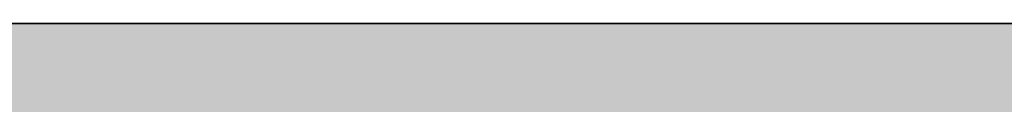
# Model space of a CAD drawing. Units: inches. Extents: x 2091 to 2899, y 967 to 2217.
# Tile 50 of 256: x 2212.145669 to 2212.151167, y 1099.918608 to 1099.919059. Entities that reach past the tile are written whole.
import ezdxf

# ---------------------------------------------------------------- set-up
doc = ezdxf.new("R2010")
doc.units = ezdxf.units.IN
doc.layers.add('A-WALL-PATT', color=141, linetype='Continuous', lineweight=13, true_color=0xadddf7)
doc.layers.add('L-SITE-WALL', color=7, linetype='Continuous', lineweight=35)

msp = doc.modelspace()

# ---------------------------------------------------------------- hatches: boundary and pattern name
at = {"layer": 'A-WALL-PATT'}
h = msp.add_hatch(color=256, dxfattribs=at)
h.dxf.hatch_style = 1
h.paths.add_polyline_path([(2212.1436027, 1941.4190588), (2387.6436027, 1941.4190588), (2387.6436027, 1824.4190588), (2392.1436027, 1824.4190588), (2392.1436027, 1941.4190588), (2609.6436027, 1941.4190588), (2609.6436027, 1825.9190588), (2614.1436027, 1825.9190588), (2614.1436027, 1941.4190588), (2794.1436027, 1941.4190588), (2794.1436027, 1928.7621663), (2803.1436027, 1928.7621663), (2803.1436027, 2050.9190588), (2203.1436027, 2050.9190588), (2203.1436027, 1900.7578592), (2212.1436027, 1900.7578592)])
h.paths.add_polyline_path([(2212.1436027, 1945.9190588), (2212.1436027, 2041.9190588), (2794.1436027, 2041.9190588), (2794.1436027, 1945.9190588), (2402.2482445, 1945.9190588), (2401.1024337, 1945.7758325), (2398.7024337, 1945.7758325)], flags=16)
h.paths.add_polyline_path([(2230.2298609, 1948.0627926), (2227.3498609, 1949.5027926), (2225.9098609, 1951.9027926), (2223.9898609, 1952.8627926), (2223.0298609, 1955.2627926), (2222.0698609, 1959.5827926), (2222.0698609, 1963.4227926), (2223.0298609, 1965.6627926), (2223.9898609, 1965.3427926), (2225.58591, 1963.860747), (2226.9115333, 1964.9572589), (2226.9488609, 1965.9387926), (2227.7783187, 1966.9521426), (2228.1999161, 1968.8787044), (2230.7098609, 1964.8627926), (2233.5898609, 1966.3027926), (2233.607309, 1966.3318728), (2233.7726595, 1964.9382048), (2234.6338015, 1963.6764729), (2235.0298609, 1963.9027926), (2236.2820348, 1965.5723578), (2235.9898609, 1962.9427926), (2237.9545121, 1957.5400019), (2238.3898609, 1957.9027926), (2239.2158609, 1960.3057926), (2238.6545655, 1966.3849599), (2238.6927918, 1966.4380694), (2238.8405779, 1967.4997069), (2238.7802908, 1967.6874864), (2238.8805378, 1967.7867629), (2238.6668609, 1966.2517926), (2239.2158609, 1960.3057926), (2238.3898609, 1957.9027926), (2236.9498609, 1956.7027926), (2234.5498609, 1949.9827926)], flags=0)
h.paths.add_polyline_path([(2278.0119735, 1948.0627926), (2276.4964266, 1947.8733492), (2275.8498328, 1947.6886081), (2274.6519735, 1947.1027926)], flags=0)
h.paths.add_polyline_path([(2269.8519735, 1955.7427926), (2268.2761762, 1956.6293287), (2270.8673022, 1956.3483982), (2269.3719735, 1958.1427926), (2268.7149641, 1959.1923253), (2270.5698328, 1958.7286081), (2268.5807252, 1961.9060872), (2270.8119735, 1960.8918835), (2270.8119735, 1963.4227926), (2271.3933148, 1964.7792556), (2270.2917623, 1966.1561963), (2271.7719735, 1965.6627926), (2272.1413868, 1966.5247568), (2273.9298328, 1965.9286081), (2275.6303855, 1968.054299), (2276.331938, 1966.72186), (2276.5204313, 1966.9521426), (2276.9420286, 1968.8787044), (2277.7342926, 1967.6110821), (2278.1398879, 1969.4645199), (2279.6591239, 1967.0337425), (2280.4119735, 1966.7827926), (2280.9493019, 1967.5887851), (2281.6098328, 1967.3686081), (2282.1332658, 1968.1537576), (2282.3492351, 1966.3334449), (2282.3498491, 1966.3325853), (2283.40755, 1968.0954201), (2283.7126314, 1965.5240203), (2284.3202211, 1964.6337894), (2284.5118085, 1964.8892393), (2284.2349735, 1965.7047926), (2284.500472, 1967.3189584), (2284.9079444, 1965.4174205), (2285.3963134, 1966.0685791), (2285.4328328, 1966.2906081), (2285.4733384, 1966.1712791), (2286.3539194, 1967.345387), (2286.2220067, 1966.1581734), (2287.6634921, 1968.0801538), (2287.7139735, 1968.4427926), (2288.4815994, 1969.0166793), (2288.5739928, 1968.7288966), (2288.9174612, 1969.0690403), (2288.6068328, 1966.8376081), (2288.9287261, 1963.3513103), (2288.9349735, 1963.3567926), (2288.9297314, 1963.3404224), (2289.015281, 1962.4138692), (2290.1112234, 1963.8751258), (2290.1328328, 1963.9426081), (2290.2176723, 1964.0170576), (2290.1112234, 1963.8751258), (2289.1558328, 1960.8916081), (2288.5940356, 1959.2572271), (2288.5719735, 1959.1027926), (2289.5319735, 1960.5427926), (2290.0119735, 1962.4627926), (2290.1918401, 1962.6426592), (2289.7698328, 1959.6886081), (2286.8898328, 1957.2886081), (2284.4898328, 1950.5686081), (2283.3146576, 1950.046308), (2283.2919735, 1949.9827926), (2280.2900585, 1948.6486081), (2281.1298328, 1948.6486081), (2282.5698328, 1948.1686081), (2283.2047262, 1948.0627926), (2278.9719735, 1948.0627926), (2276.0919735, 1949.5027926), (2274.6519735, 1951.9027926), (2272.7319735, 1952.8627926)], flags=0)
h.paths.add_polyline_path([(2271.1588684, 1958.0217654), (2272.9698328, 1955.8486081), (2272.0098328, 1960.1686081), (2272.0098328, 1964.0086081), (2272.6244258, 1965.4426583), (2274.3280226, 1963.860747), (2275.6536458, 1964.9572589), (2275.6377429, 1964.5390903), (2277.4122311, 1966.0068885), (2277.0329735, 1965.1567926), (2276.829924, 1964.9755966), (2276.7660116, 1963.2950136), (2277.4496351, 1962.6602203), (2279.4519735, 1964.8627926), (2282.3319735, 1966.3027926), (2283.5298328, 1966.8886081), (2283.2945117, 1966.7709476), (2283.9129934, 1963.8846999), (2284.8992493, 1964.4482747), (2284.7319735, 1962.9427926), (2286.6966247, 1957.5400019), (2287.1319735, 1957.9027926), (2287.5419128, 1959.0953883), (2287.7793955, 1958.4423109), (2285.6827383, 1956.6950966), (2285.8765033, 1959.7953357), (2284.7319735, 1962.9427926), (2284.8992493, 1964.4482747), (2283.9129934, 1963.8846999), (2284.2238328, 1962.4341157), (2283.4243649, 1963.6054836), (2281.6098328, 1962.5686081), (2281.1298328, 1960.1686081), (2282.0898328, 1956.3286081), (2283.0498328, 1952.9686081), (2282.5698328, 1950.5686081), (2280.1698328, 1948.6486081), (2279.883316, 1948.7918666), (2278.9719735, 1948.0627926), (2278.9719735, 1949.0227926), (2278.6723132, 1949.3973679), (2277.2898328, 1950.0886081), (2275.8498328, 1952.4886081), (2273.9298328, 1953.4486081), (2272.4898328, 1954.8886081), (2271.9216473, 1954.8886081), (2271.7719735, 1955.2627926)], flags=0)
h.paths.add_polyline_path([(2311.994146, 1955.7427926), (2312.0627174, 1955.6742211), (2312.0550999, 1955.7085002)], flags=0)
h.paths.add_polyline_path([(2331.956146, 1963.9517926), (2333.396146, 1965.3917926), (2331.077146, 1963.3567926), (2330.998603, 1963.1115166)], flags=0)
h.paths.add_polyline_path([(2310.554146, 1954.3027926), (2307.0398066, 1956.2799434), (2310.7629029, 1955.8762843), (2312.474146, 1953.8227926), (2313.434146, 1951.4227926), (2315.354146, 1950.4627926), (2316.794146, 1948.0627926), (2317.466146, 1947.7267926), (2319.3686915, 1947.9646108), (2317.754146, 1949.9827926), (2317.5695306, 1950.6104849), (2316.794146, 1951.9027926), (2314.874146, 1952.8627926), (2313.914146, 1955.2627926), (2311.514146, 1958.1427926), (2309.3754889, 1961.5591681), (2311.514146, 1960.3370783), (2311.514146, 1961.9827926), (2310.6046723, 1963.1196347), (2311.726605, 1962.4785303), (2312.4183321, 1964.09256), (2312.2559642, 1964.2955198), (2313.194146, 1963.9827926), (2313.914146, 1965.6627926), (2314.6467776, 1965.418582), (2315.354146, 1966.3027926), (2316.794146, 1967.7427926), (2316.1574354, 1966.9469043), (2317.0341105, 1965.28186), (2317.2226038, 1965.5121426), (2317.7770481, 1968.0457711), (2318.4741105, 1966.72186), (2318.6626038, 1966.9521426), (2319.0842012, 1968.8787044), (2321.2070492, 1965.4821474), (2322.1614187, 1966.9137017), (2322.554146, 1966.7827926), (2322.7859877, 1967.1305552), (2322.881646, 1966.3242926), (2323.3120408, 1965.7217399), (2323.6512889, 1965.891364), (2324.3964998, 1967.1333822), (2324.6569446, 1964.9382048), (2324.971986, 1964.476611), (2325.3872804, 1967.001499), (2325.9408127, 1964.4183481), (2327.2289286, 1966.1358361), (2327.1663199, 1965.5723578), (2328.0591386, 1966.7627827), (2328.2245759, 1966.2474864), (2329.6679714, 1967.6769101), (2329.6645759, 1967.6874864), (2329.7648229, 1967.7867629), (2329.551146, 1966.2517926), (2330.100146, 1960.3057926), (2329.3328143, 1958.0734703), (2329.3130649, 1957.935225), (2329.634146, 1958.2027926), (2330.234146, 1959.1027926), (2330.714146, 1961.0227926), (2331.034146, 1961.3427926), (2330.714146, 1959.1027926), (2329.634146, 1958.2027926), (2329.274146, 1957.6627926), (2327.7121121, 1956.3610977), (2325.434146, 1949.9827926), (2324.3337687, 1949.493736), (2323.994146, 1948.5427926), (2319.674146, 1946.6227926), (2316.794146, 1948.0627926), (2315.354146, 1950.4627926), (2313.434146, 1951.4227926)], flags=0)
h.paths.add_polyline_path([(2321.3356845, 1947.9520233), (2321.114146, 1948.0627926), (2321.114146, 1949.0227926), (2319.194146, 1951.4227926), (2316.794146, 1959.5827926), (2316.6632369, 1959.5827926), (2315.354146, 1958.1427926), (2314.394146, 1958.1427926), (2313.1483033, 1958.7090847), (2312.954146, 1959.5827926), (2312.954146, 1960.8918835), (2315.834146, 1959.5827926), (2316.6632369, 1959.5827926), (2317.3147094, 1960.2994123), (2315.0301951, 1962.420747), (2316.3558184, 1963.5172589), (2316.3723369, 1963.9516153), (2316.4701951, 1963.860747), (2317.7958184, 1964.9572589), (2317.7552187, 1963.8896871), (2319.175146, 1965.1567926), (2319.4984065, 1965.8813724), (2321.114146, 1965.3427926), (2323.2358851, 1962.3723578), (2325.6863494, 1963.7726231), (2325.5427886, 1962.4805756), (2325.1987827, 1963.4940135), (2324.4785097, 1963.0824289), (2324.9260053, 1960.9941157), (2324.0780866, 1962.2364729), (2322.4147912, 1961.2860184), (2322.074146, 1959.5827926), (2323.034146, 1955.7427926), (2323.994146, 1952.3827926), (2323.514146, 1949.9827926), (2322.1427174, 1948.8856497), (2322.074146, 1948.5427926)], flags=0)
h.paths.add_polyline_path([(2320.2074794, 1963.3374592), (2320.154146, 1963.4227926), (2320.394146, 1963.5427926)], flags=0)
h.paths.add_polyline_path([(2353.8505274, 1965.8105004), (2354.0305274, 1965.7505004), (2354.3305274, 1966.4505004), (2354.3305274, 1966.9305004)], flags=0)
h.paths.add_polyline_path([(2359.0205825, 1969.0264122), (2359.0983824, 1968.9019323), (2359.2335274, 1969.5195004), (2359.2335274, 1969.9995004)], flags=0)
h.paths.add_polyline_path([(2358.2566937, 1966.6816724), (2357.983601, 1966.3480346), (2358.211267, 1966.1461745), (2358.4104918, 1966.3895678)], flags=0)
h.paths.add_polyline_path([(2357.7684731, 1966.0587777), (2357.7321997, 1965.1049667), (2357.751047, 1965.1205565), (2357.7695274, 1965.6065004), (2357.7695274, 1966.057843)], flags=0)
h.paths.add_polyline_path([(2359.1115274, 1965.3045004), (2359.1115274, 1964.8245004), (2359.8445274, 1966.4675004), (2359.8445274, 1966.9475004)], flags=0)
h.paths.add_polyline_path([(2360.2236843, 1966.6214493), (2360.6985274, 1969.3625004), (2360.6985274, 1969.8425004), (2360.2105274, 1967.0255004), (2360.2105274, 1966.6425004)], flags=0)
h.paths.add_polyline_path([(2363.4505274, 1967.8905004), (2363.4505274, 1968.3705004), (2362.4905274, 1966.9305004), (2362.6560446, 1966.6987763)], flags=0)
h.paths.add_polyline_path([(2364.4755226, 1966.0788259), (2365.8505274, 1968.3705004), (2365.8505274, 1968.8505004), (2364.4279755, 1966.4795806)], flags=0)
h.paths.add_polyline_path([(2366.3135274, 1965.8525004), (2366.3667086, 1965.6958291), (2366.8025274, 1968.3455004), (2366.8025274, 1968.8255004)], flags=0)
h.paths.add_polyline_path([(2367.16531, 1965.8035439), (2367.2905274, 1966.9305004), (2367.2905274, 1967.4105004), (2367.1027013, 1965.7200656)], flags=0)
h.paths.add_polyline_path([(2370.0365274, 1959.9735004), (2371.0135274, 1963.0245004), (2371.0135274, 1963.5045004), (2370.0365274, 1960.4535004)], flags=0)
h.paths.add_polyline_path([(2371.6105274, 1960.2105004), (2372.5705274, 1961.6505004), (2372.5705274, 1962.1305004), (2371.8025274, 1960.9785004)], flags=0)
h.paths.add_polyline_path([(2350.8736661, 1956.0050856), (2351.9305274, 1955.8905004), (2354.4905274, 1953.3305004), (2353.8505274, 1954.9305004), (2351.4505274, 1957.8105004), (2347.9355274, 1963.4255004), (2347.9355274, 1963.9055004), (2351.4505274, 1958.2905004), (2353.7050728, 1955.5850458), (2352.8905274, 1959.2505004), (2352.8905274, 1959.7305004), (2352.8905274, 1961.9247861), (2356.7305274, 1959.7305004), (2358.454471, 1961.6268384), (2354.8105274, 1965.0105004), (2355.0308552, 1965.2859102), (2358.6910907, 1961.8871201), (2361.5305274, 1965.0105004), (2364.3764954, 1966.4334844), (2364.5243939, 1965.1869106), (2365.454468, 1963.8241807), (2365.8810728, 1964.0679549), (2365.3705274, 1966.4505004), (2365.3705274, 1966.9305004), (2366.8105274, 1960.2105004), (2366.8105274, 1959.7305004), (2366.3887092, 1952.9814095), (2367.7705274, 1956.8505004), (2368.641225, 1957.5760818), (2366.8105274, 1962.6105004), (2366.8105274, 1963.0905004), (2368.7751785, 1957.6877097), (2369.2105274, 1958.0505004), (2370.0015924, 1960.3518674), (2369.4752319, 1966.0526677), (2369.5134582, 1966.1057772), (2369.514173, 1966.1109121), (2369.4752319, 1966.5326677), (2369.5134582, 1966.5857772), (2369.614635, 1967.3125914), (2369.1825274, 1968.6585004), (2369.1825274, 1969.1385004), (2369.6009573, 1967.8351942), (2369.7012042, 1967.9344708), (2369.7179468, 1968.054743), (2370.1451758, 1968.3741448), (2369.7787075, 1968.0112238), (2369.7012042, 1967.4544708), (2370.4681613, 1968.2140038), (2369.674936, 1967.2657706), (2369.514173, 1966.1109121), (2370.0365274, 1960.4535004), (2370.0365274, 1959.9735004), (2369.441756, 1958.2431909), (2370.6505274, 1959.2505004), (2371.0458215, 1962.0175592), (2371.1305274, 1962.1305004), (2370.6505274, 1958.7705004), (2367.7705274, 1956.3705004), (2365.3705274, 1949.6505004), (2362.0790988, 1948.1876432), (2363.4505274, 1947.7305004), (2361.0505274, 1947.7305004), (2360.0905274, 1947.7305004), (2357.1038607, 1947.3571671), (2360.0905274, 1948.2105004), (2358.1705274, 1949.1705004), (2356.7305274, 1951.5705004), (2354.8105274, 1952.5305004), (2351.9305274, 1955.4105004)], flags=0)
h.paths.add_polyline_path([(2361.0505274, 1948.6905004), (2359.1305274, 1951.0905004), (2356.7305274, 1959.2505004), (2355.7705274, 1959.2505004), (2352.8905274, 1960.5595913), (2352.8905274, 1961.4447861), (2355.8905274, 1959.7305004), (2356.7305274, 1959.7305004), (2356.837194, 1959.3678337), (2361.5305274, 1964.5305004), (2363.2484221, 1965.3894478), (2364.92531, 1963.0418047), (2362.4905274, 1961.6505004), (2362.0638607, 1959.5171671), (2362.9705274, 1955.8905004), (2363.9305274, 1952.5305004), (2363.9305274, 1952.0505004), (2363.4505274, 1949.6505004), (2361.0505274, 1947.7305004)], flags=0)
h.paths.add_polyline_path([(2359.1305274, 1951.5705004), (2359.2905274, 1951.3705004), (2361.0505274, 1954.4505004), (2361.0505274, 1954.9305004)], flags=0)
h.paths.add_polyline_path([(2357.2195274, 1966.5455004), (2356.7925274, 1968.8145004), (2356.7925274, 1969.2945004), (2357.2195274, 1967.0255004)], flags=0)
h.paths.add_polyline_path([(2361.0505274, 1954.4505004), (2361.5305274, 1958.7705004), (2361.5305274, 1959.2505004), (2361.0505274, 1954.9305004)], flags=0)
h.paths.add_polyline_path([(2402.5482874, 1948.4860764), (2402.3024337, 1948.4158325), (2402.5904337, 1948.4158325)], flags=0)
h.paths.add_polyline_path([(2394.1424337, 1956.0958325), (2395.6850518, 1954.5532144), (2396.7204952, 1953.9706788), (2396.0624337, 1955.6158325), (2395.2413811, 1956.6010956), (2395.8789043, 1956.4417148), (2395.1024337, 1959.9358325), (2395.1024337, 1963.7758325), (2396.0624337, 1966.0158325), (2397.0224337, 1965.6958325), (2398.6184828, 1964.2137869), (2399.9441061, 1965.3102988), (2399.9814337, 1966.2918325), (2400.8108915, 1967.3051825), (2401.2324888, 1969.2317443), (2403.5379492, 1965.5430077), (2403.9419843, 1967.3893156), (2404.7024337, 1967.1358325), (2405.4603284, 1966.0747799), (2406.6224337, 1966.6558325), (2406.6398818, 1966.6849127), (2406.8052323, 1965.2912447), (2406.9256943, 1965.1147456), (2407.3424337, 1964.9758325), (2407.8743256, 1965.7736703), (2408.1691004, 1964.3980547), (2409.3146076, 1965.9253977), (2409.2174583, 1965.0510538), (2409.4452323, 1963.1312447), (2410.3063743, 1961.8695128), (2410.7024337, 1962.0958325), (2411.4422687, 1963.0822792), (2411.1654337, 1963.8978325), (2411.6164263, 1966.6397566), (2411.7253645, 1966.7911093), (2411.8731507, 1967.8527468), (2411.8128636, 1968.0405263), (2411.9131106, 1968.1398028), (2411.6994337, 1966.6048325), (2412.2484337, 1960.6588325), (2413.2254337, 1963.7098325), (2414.3779002, 1964.7211603), (2414.5131507, 1965.6927468), (2414.4528636, 1965.8805263), (2414.5531106, 1965.9798028), (2414.3779002, 1964.7211603), (2414.5198172, 1964.8456973), (2414.3653645, 1964.6311093), (2414.3394337, 1964.4448325), (2414.8884337, 1958.4988325), (2414.0624337, 1956.0958325), (2412.6224337, 1954.8958325), (2410.1713699, 1948.0328538), (2410.0167194, 1948.0844039), (2405.9024337, 1946.2558325), (2405.9024337, 1947.2158325), (2405.2042519, 1948.0885598), (2404.2224337, 1948.4158325), (2403.2624337, 1948.4158325), (2400.3824337, 1949.8558325), (2399.6624337, 1951.0558325), (2397.9824337, 1952.7358325), (2397.0224337, 1953.2158325), (2395.6850518, 1954.5532144), (2392.6567764, 1956.2569078)], flags=0)
h.paths.add_polyline_path([(2409.0856501, 1964.4074407), (2409.1303635, 1964.2757154), (2409.2624337, 1964.4958325)], flags=0)
h.paths.add_polyline_path([(2397.7424337, 1961.6158325), (2398.7024337, 1963.8558325), (2399.6624337, 1963.5358325), (2401.4265631, 1965.7409942), (2401.7914151, 1966.5588003), (2402.0714337, 1965.0708325), (2402.8355074, 1964.3933667), (2403.2623982, 1964.9148999), (2403.3381187, 1964.771086), (2402.6155159, 1963.9762229), (2402.4986125, 1960.9022379), (2403.5429971, 1959.9324522), (2404.4132029, 1960.8896786), (2404.7024337, 1962.3358325), (2407.9163468, 1964.1723542), (2409.5202115, 1961.9269436), (2410.9870849, 1957.8930418), (2411.4224337, 1958.2558325), (2412.0479637, 1960.075625), (2412.4103407, 1959.0790883), (2411.6756205, 1958.4668215), (2411.6624337, 1958.2558325), (2411.6260701, 1958.4255295), (2409.9824337, 1957.0558325), (2407.5824337, 1950.3358325), (2403.2624337, 1948.4158325), (2403.2624337, 1949.3758325), (2401.3424337, 1951.7758325), (2399.4165078, 1958.3239806), (2397.7424337, 1959.0849234), (2397.7424337, 1959.9701182), (2397.1024337, 1960.3358325), (2397.7424337, 1960.0449234)], flags=0)
h.paths.add_polyline_path([(2405.9024337, 1952.9758325), (2405.9504337, 1953.4078325), (2406.0167194, 1953.1758325)], flags=0)
h.paths.add_polyline_path([(2449.817778, 1967.1140143), (2449.7523235, 1967.1358325), (2449.7937028, 1967.0779014)], flags=0)
h.paths.add_polyline_path([(2451.6976961, 1966.6181202), (2451.7408949, 1966.6901182), (2451.6920515, 1966.6656965)], flags=0)
h.paths.add_polyline_path([(2454.3436278, 1965.7375716), (2455.7523235, 1967.6158325), (2455.9923235, 1968.0958325), (2454.3644974, 1965.9253977)], flags=0)
h.paths.add_polyline_path([(2457.5473235, 1968.8638325), (2457.7873235, 1969.3438325), (2457.0543235, 1968.7958325), (2457.0076216, 1968.4603446)], flags=0)
h.paths.add_polyline_path([(2456.9217835, 1967.8566619), (2456.8022381, 1968.2290163), (2456.7230003, 1967.6598028)], flags=0)
h.paths.add_polyline_path([(2457.3023235, 1967.3768325), (2457.5423235, 1967.8568325), (2456.8103235, 1966.8398325), (2456.7405164, 1966.7002183), (2456.7490213, 1966.6081053)], flags=0)
h.paths.add_polyline_path([(2458.2753235, 1963.7098325), (2458.1553426, 1963.3351533), (2460.3543235, 1965.2648325), (2460.5943235, 1965.7448325)], flags=0)
h.paths.add_polyline_path([(2458.3923235, 1962.8158325), (2458.3640882, 1962.6181854), (2459.5923235, 1964.2558325), (2459.8323235, 1964.7358325)], flags=0)
h.paths.add_polyline_path([(2459.3523235, 1962.8158325), (2459.2723235, 1962.4958325), (2460.0723235, 1963.2958325), (2460.3123235, 1963.7758325)], flags=0)
h.paths.add_polyline_path([(2458.6803235, 1960.6078325), (2458.6323235, 1960.4158325), (2459.5923235, 1961.8558325), (2459.8323235, 1962.3358325)], flags=0)
h.paths.add_polyline_path([(2437.8381696, 1956.2426502), (2439.1923235, 1956.0958325), (2441.3523235, 1953.9358325), (2440.8723235, 1955.1358325), (2438.4723235, 1958.0158325), (2438.0715634, 1958.6560225), (2438.7123235, 1958.4958325), (2440.6395962, 1956.1831052), (2439.9123235, 1959.4558325), (2439.9123235, 1963.2958325), (2441.3523235, 1966.6558325), (2441.5923235, 1967.1358325), (2441.1123235, 1966.0158325), (2442.0723235, 1965.6958325), (2443.9889932, 1968.0916696), (2444.2413235, 1966.7508325), (2444.9168011, 1966.1519203), (2445.6765737, 1967.0801359), (2446.2553235, 1969.7248325), (2446.4953235, 1970.2048325), (2446.2823786, 1969.2317443), (2447.362672, 1967.5032748), (2447.7203235, 1969.5678325), (2447.9603235, 1970.0478325), (2447.4854804, 1967.3067814), (2448.7923235, 1965.2158325), (2448.4723235, 1964.8638325), (2448.5523235, 1964.7358325), (2451.4520515, 1966.1856965), (2451.615122, 1964.8112447), (2452.3079173, 1963.7961718), (2453.2345053, 1964.3256507), (2454.0723235, 1960.4158325), (2453.6286871, 1953.3176507), (2454.7923235, 1956.5758325), (2455.0323235, 1957.0558325), (2455.7188351, 1957.6279255), (2453.8323235, 1962.8158325), (2453.940966, 1963.7936155), (2453.3353235, 1965.5778325), (2453.8243235, 1968.5508325), (2454.0643235, 1969.0308325), (2453.5753235, 1966.0578325), (2454.0403331, 1964.6879188), (2453.8323235, 1962.8158325), (2455.7188351, 1957.6279255), (2456.3672068, 1958.1682353), (2457.0583235, 1960.1788325), (2457.2983235, 1960.6588325), (2456.4723235, 1958.2558325), (2457.7177289, 1959.2936703), (2457.6723235, 1958.9758325), (2454.8899506, 1956.6571884), (2453.6141416, 1953.0849234), (2453.5923235, 1952.7358325), (2453.3523235, 1952.2558325), (2453.3595962, 1952.3721961), (2452.6323235, 1950.3358325), (2452.3923235, 1949.8558325), (2449.203752, 1948.4386896), (2450.7123235, 1947.9358325), (2448.0723235, 1947.9358325), (2447.1123235, 1947.9358325), (2444.5523235, 1947.6158325), (2447.1995962, 1948.3721961), (2445.1923235, 1949.3758325), (2443.7523235, 1951.7758325), (2441.8323235, 1952.7358325), (2438.9523235, 1955.6158325)], flags=0)
h.paths.add_polyline_path([(2443.9923235, 1959.9358325), (2444.0403235, 1959.7726325), (2444.1215542, 1959.8619863)], flags=0)
h.paths.add_polyline_path([(2442.9123235, 1959.9358325), (2443.0323235, 1959.9358325), (2442.4456568, 1960.2024992)], flags=0)
h.paths.add_polyline_path([(2444.9829435, 1965.0196767), (2445.2793235, 1965.2648325), (2445.5193235, 1965.7448325), (2444.9939958, 1965.3102988)], flags=0)
h.paths.add_polyline_path([(2446.1333235, 1965.0298325), (2446.3303662, 1965.4714986), (2444.9703235, 1964.2578325), (2444.7303235, 1963.7778325)], flags=0)
h.paths.add_polyline_path([(2442.7923235, 1959.4558325), (2443.7523235, 1959.4558325), (2446.1523235, 1951.2958325), (2446.4123235, 1951.7508325), (2446.3923235, 1951.7758325), (2448.0805993, 1954.7303152), (2448.5523235, 1958.9758325), (2441.8323235, 1965.2158325), (2442.1549464, 1965.6191112), (2448.7923235, 1959.4558325), (2448.3123235, 1955.1358325), (2448.0723235, 1954.6558325), (2446.4123235, 1951.7508325), (2448.3123235, 1949.3758325), (2448.3123235, 1948.4158325), (2450.5408949, 1950.1986896), (2450.9523235, 1952.2558325), (2449.9923235, 1955.6158325), (2449.0323235, 1959.4558325), (2449.5123235, 1961.8558325), (2449.7523235, 1962.3358325), (2449.6749041, 1961.9487357), (2452.9945053, 1963.8456507), (2453.0644143, 1963.5194086), (2452.8846108, 1963.7828538), (2449.6749041, 1961.9487357), (2449.2723235, 1959.9358325), (2450.2323235, 1956.0958325), (2451.1923235, 1952.7358325), (2450.7123235, 1950.3358325), (2450.4723235, 1949.8558325), (2448.0723235, 1947.9358325), (2448.0723235, 1948.5358325), (2445.4323235, 1949.8558325), (2443.9923235, 1952.2558325), (2442.0723235, 1953.2158325), (2441.1123235, 1955.6158325), (2440.1523235, 1959.9358325), (2440.1523235, 1960.6558325)], flags=0)
h.paths.add_polyline_path([(2456.6923235, 1966.9858325), (2457.6083235, 1968.0808325), (2457.8483235, 1968.5608325), (2456.9323235, 1967.4658325)], flags=0)
h.paths.add_polyline_path([(2489.8965704, 1966.5802407), (2489.9429477, 1966.1893466), (2490.7474884, 1967.5302478), (2491.3191223, 1968.9511605)], flags=0)
h.paths.add_polyline_path([(2473.5624709, 1956.4071313), (2477.139981, 1956.0192567), (2476.955333, 1956.2408343), (2475.1080486, 1957.2801078), (2476.3474884, 1956.9702478), (2475.1869011, 1958.8242158), (2476.9191223, 1958.3911605), (2475.4116422, 1960.7992688), (2477.7874884, 1959.7193388), (2477.7874884, 1962.2502478), (2477.637399, 1962.4378595), (2477.8225502, 1962.3320588), (2478.3591223, 1963.5840603), (2478.3591223, 1963.6711605), (2477.3243485, 1964.9646278), (2478.7148258, 1964.5011354), (2479.3191223, 1965.9111605), (2480.2791223, 1965.5911605), (2481.7839654, 1967.4722144), (2482.1164884, 1965.7052478), (2482.8805621, 1965.027782), (2483.209305, 1965.4294079), (2483.2201695, 1965.7150902), (2483.0759397, 1965.9890218), (2483.7117624, 1966.7658076), (2484.1304884, 1968.6792478), (2484.7021223, 1970.1001605), (2484.4891774, 1969.1270723), (2486.5029044, 1965.9051092), (2487.3874884, 1965.6102478), (2488.1534195, 1966.7591445), (2488.717017, 1965.9701079), (2489.2000857, 1966.2116422), (2489.3306713, 1965.1109919), (2490.3939049, 1963.6224649), (2490.6607651, 1963.7749564), (2490.4939052, 1964.553636), (2490.9230629, 1963.9248409), (2491.3191223, 1964.1511605), (2491.3333892, 1964.1701831), (2491.2104884, 1964.5322478), (2491.2817559, 1964.9655369), (2491.425789, 1964.2933827), (2494.0764757, 1967.8276317), (2494.4979183, 1966.5149416), (2494.5981652, 1966.6142182), (2494.6894884, 1967.2702478), (2495.106748, 1967.5821964), (2495.1298393, 1967.7480749), (2495.0695522, 1967.9358543), (2495.1697991, 1968.0351309), (2495.0317768, 1967.0436325), (2495.7538179, 1967.7586844), (2494.9820531, 1966.6864374), (2494.9561223, 1966.5001605), (2495.4790212, 1960.8368513), (2495.9104884, 1962.1842478), (2496.4821223, 1963.6051605), (2496.0726945, 1962.3265891), (2496.7689042, 1962.9375364), (2496.5991223, 1962.7111605), (2496.1191223, 1959.3511605), (2496.7328731, 1960.2717868), (2496.9874884, 1961.2902478), (2497.5591223, 1962.7111605), (2497.0791223, 1960.7911605), (2496.5074884, 1959.3702478), (2495.5474884, 1957.9302478), (2492.7588421, 1955.6063759), (2490.8391223, 1950.2311605), (2490.2674884, 1948.8102478), (2485.9474884, 1946.8902478), (2483.0674884, 1948.3302478), (2481.6274884, 1950.7302478), (2479.7074884, 1951.6902478), (2476.8274884, 1954.5702478)], flags=0)
h.paths.add_polyline_path([(2485.5769732, 1948.3133919), (2485.5591223, 1948.3111605), (2485.5787582, 1948.3111605)], flags=0)
h.paths.add_polyline_path([(2478.6450633, 1954.5511605), (2478.1090419, 1956.963257), (2479.3191223, 1955.5111605), (2480.2791223, 1953.1111605), (2482.1991223, 1952.1511605), (2483.6391223, 1949.7511605), (2486.5191223, 1948.3111605), (2486.5191223, 1949.2711605), (2484.7393067, 1951.49593), (2484.0274884, 1950.2502478), (2481.6274884, 1958.4102478), (2482.3751479, 1959.2326733), (2482.1991223, 1959.8311605), (2483.1975724, 1960.9294556), (2479.7074884, 1964.1702478), (2480.6033578, 1965.2900847), (2481.8751714, 1964.109115), (2482.666387, 1964.7635825), (2482.6153591, 1963.4217978), (2482.9891988, 1963.0746609), (2484.0084884, 1963.9842478), (2484.6836065, 1965.4975071), (2484.5801223, 1965.4051605), (2485.3572683, 1967.1471126), (2485.1206453, 1965.7811968), (2486.4274884, 1963.6902478), (2488.1453831, 1964.5491952), (2489.822271, 1962.2015522), (2490.7474884, 1962.7302478), (2491.9996623, 1964.3998131), (2492.0760458, 1965.0872647), (2492.2128915, 1964.6841187), (2492.4853744, 1965.0474291), (2492.2791223, 1963.1911605), (2494.2437735, 1957.7883698), (2494.5625035, 1958.0539782), (2494.9334884, 1959.1332478), (2495.5051223, 1960.5541605), (2494.6791223, 1958.1511605), (2494.1074884, 1956.7302478), (2494.5625035, 1958.0539782), (2493.4085439, 1957.0923452), (2491.7074884, 1961.7702478), (2491.9996623, 1964.3998131), (2490.7474884, 1962.7302478), (2487.7120303, 1960.9957003), (2487.4791223, 1959.8311605), (2488.4391223, 1955.9911605), (2489.3991223, 1952.6311605), (2488.9191223, 1950.2311605), (2488.5769183, 1949.9573973), (2488.3474884, 1948.8102478), (2487.6517154, 1948.2536295), (2487.4791223, 1948.3111605), (2486.5191223, 1948.3111605), (2483.6391223, 1949.7511605), (2482.1991223, 1952.1511605), (2480.2791223, 1953.1111605), (2478.8391223, 1954.5511605)], flags=0)
h.paths.add_polyline_path([(2526.648252, 1966.9875242), (2526.5173429, 1967.0311605), (2526.6001016, 1966.9152985)], flags=0)
h.paths.add_polyline_path([(2528.4706401, 1966.4466558), (2528.5744858, 1966.619732), (2528.4570709, 1966.5610245)], flags=0)
h.paths.add_polyline_path([(2534.1333429, 1967.4961605), (2534.1566852, 1967.5428451), (2534.0598415, 1967.4082958)], flags=0)
h.paths.add_polyline_path([(2536.1619229, 1964.0506005), (2535.1573429, 1962.7111605), (2535.1008723, 1962.3158664), (2536.1173429, 1963.6711605), (2536.4205319, 1964.2775386)], flags=0)
h.paths.add_polyline_path([(2535.1573429, 1959.8311605), (2536.1173429, 1961.2711605), (2536.5973429, 1962.2311605), (2535.2533429, 1960.2151605)], flags=0)
h.paths.add_polyline_path([(2513.2490352, 1956.284796), (2516.2211807, 1955.9625552), (2514.9973429, 1957.4311605), (2514.1958227, 1958.7115406), (2515.4773429, 1958.3911605), (2516.9318884, 1956.645706), (2516.4373429, 1958.8711605), (2516.4373429, 1962.7111605), (2516.8726918, 1963.7269745), (2515.3464338, 1965.6347969), (2517.3973429, 1964.9511605), (2517.8773429, 1966.0711605), (2518.3573429, 1967.0311605), (2517.8773429, 1965.9111605), (2518.8373429, 1965.5911605), (2520.4865896, 1967.6527188), (2520.7663429, 1966.1661605), (2521.5304166, 1965.4886947), (2521.7814433, 1965.7953745), (2521.8009106, 1966.307268), (2521.4778037, 1966.9209358), (2521.2463429, 1967.1261605), (2521.1777006, 1967.4909132), (2521.4778037, 1966.9209358), (2522.0104166, 1966.4486947), (2522.2573857, 1966.7504173), (2522.7803429, 1969.1401605), (2523.2603429, 1970.1001605), (2523.0473981, 1969.1270723), (2524.6731324, 1966.5258974), (2526.0373429, 1966.0711605), (2526.7952377, 1965.0101079), (2527.9770709, 1965.6010245), (2528.1401415, 1964.2265727), (2528.6645901, 1963.4581589), (2529.3886157, 1963.8718878), (2529.3296653, 1964.1469896), (2529.4812835, 1963.9248409), (2529.8773429, 1964.1511605), (2529.9840096, 1964.2933827), (2529.7890531, 1965.2031796), (2530.0623998, 1964.397903), (2532.802483, 1968.0513473), (2533.1477728, 1966.9758543), (2533.2480198, 1967.0751309), (2533.3393429, 1967.7311605), (2533.6728477, 1967.9804929), (2533.7280198, 1968.0351309), (2533.5143429, 1966.5001605), (2534.0247176, 1960.9724963), (2534.5603429, 1962.6451605), (2535.0403429, 1963.6051605), (2534.0633429, 1960.5541605), (2533.2373429, 1958.1511605), (2534.2881537, 1959.0268362), (2534.1973429, 1958.3911605), (2531.5125972, 1956.1538724), (2529.3973429, 1950.2311605), (2528.9173429, 1949.2711605), (2526.4487715, 1948.1740177), (2527.4773429, 1947.8311605), (2530.3573429, 1947.3511605), (2524.5973429, 1947.3511605), (2521.7173429, 1948.7911605), (2520.2773429, 1951.1911605), (2518.3573429, 1952.1511605), (2515.4773429, 1955.0311605)], flags=0)
h.paths.add_polyline_path([(2523.9347601, 1967.1903084), (2523.6195125, 1966.4836893), (2523.7704999, 1966.2421094)], flags=0)
h.paths.add_polyline_path([(2518.8373429, 1953.1111605), (2517.8773429, 1955.5111605), (2516.8849834, 1959.9767785), (2516.9173429, 1959.9620696), (2516.9173429, 1962.0254462), (2520.7573429, 1959.8311605), (2522.0249486, 1961.2255267), (2518.3573429, 1964.6311605), (2519.0025888, 1965.4377179), (2520.433392, 1964.109115), (2521.3011199, 1964.8268709), (2521.2451575, 1963.3553327), (2525.6383068, 1959.2759798), (2526.0373429, 1961.2711605), (2529.3973429, 1963.1911605), (2530.6495168, 1964.8607257), (2530.6647196, 1964.9975502), (2530.6919561, 1964.9173115), (2531.0877777, 1965.4450736), (2530.9459855, 1964.1689435), (2530.6919561, 1964.9173115), (2529.3973429, 1963.1911605), (2526.3625042, 1961.456967), (2526.0373429, 1959.8311605), (2526.9973429, 1955.9911605), (2527.9573429, 1952.6311605), (2527.4773429, 1950.2311605), (2527.1344858, 1949.9568748), (2526.9739283, 1949.1540874), (2526.6973429, 1949.0311605), (2524.5973429, 1947.3511605), (2524.5973429, 1948.3111605), (2524.2773429, 1948.7111605), (2522.1973429, 1949.7511605), (2520.7573429, 1952.1511605)], flags=0)
h.paths.add_polyline_path([(2520.2773429, 1958.8711605), (2520.8533429, 1959.5047605), (2523.1573429, 1951.6711605), (2524.6138947, 1954.220126), (2524.5973429, 1954.0711605), (2522.6773429, 1950.7111605)], flags=0)
h.paths.add_polyline_path([(2559.3709104, 1966.3111605), (2559.3984114, 1966.324911), (2559.4019428, 1966.3452961)], flags=0)
h.paths.add_polyline_path([(2549.7709104, 1957.1911605), (2552.6509104, 1954.3111605), (2552.1339874, 1955.6034682), (2550.6109104, 1957.4311605), (2547.0959104, 1963.0461605), (2545.7759104, 1965.2061605), (2549.2909104, 1959.5911605), (2551.6909104, 1956.7111605), (2550.7929329, 1960.7520594), (2550.7309104, 1960.7802514), (2550.7309104, 1964.8711605), (2551.6909104, 1967.1111605), (2552.6509104, 1966.7911605), (2554.2469595, 1965.309115), (2555.0342517, 1965.9603371), (2555.5816714, 1966.6446117), (2555.6099104, 1967.3871605), (2556.4393682, 1968.4005106), (2556.8609656, 1970.3270723), (2559.3709104, 1966.3111605), (2560.6909104, 1964.1511605), (2562.4088052, 1965.0101079), (2561.6509104, 1966.0711605), (2560.3309104, 1968.2311605), (2561.7584966, 1966.2325398), (2562.3472126, 1967.1156138), (2562.433709, 1966.3865727), (2563.127798, 1965.3696043), (2563.5709104, 1965.5911605), (2563.5883585, 1965.6202407), (2563.3625433, 1967.5235403), (2563.7224894, 1965.8437921), (2565.0600013, 1968.0729787), (2564.7328616, 1965.1287215), (2565.1175771, 1963.3333827), (2567.4446216, 1966.4361087), (2567.315615, 1967.8333279), (2567.3538413, 1967.8864374), (2567.5016274, 1968.9480749), (2567.4413403, 1969.1358543), (2567.5415873, 1969.2351309), (2567.3279104, 1967.7001605), (2567.8769104, 1961.7541605), (2568.7466892, 1964.4703273), (2568.635615, 1965.6733279), (2568.6738413, 1965.7264374), (2568.8216274, 1966.7880749), (2568.7613403, 1966.9758543), (2568.8615873, 1967.0751309), (2568.6479104, 1965.5401605), (2568.7261271, 1964.6930264), (2568.8539104, 1964.8051605), (2568.7466892, 1964.4703273), (2568.8172361, 1963.7062615), (2568.9709104, 1963.9111605), (2568.8660747, 1963.1773104), (2569.1969104, 1959.5941605), (2568.3709104, 1957.1911605), (2566.9309104, 1955.9911605), (2564.6202721, 1949.5213733), (2564.6509104, 1949.5111605), (2564.6166247, 1949.5111605), (2564.5309104, 1949.2711605), (2560.2109104, 1947.3511605), (2557.3309104, 1948.7911605), (2556.0451961, 1950.9340177), (2556.0109104, 1950.9511605), (2555.8566247, 1951.2083034), (2553.9709104, 1952.1511605), (2551.0909104, 1955.0311605), (2546.6501439, 1957.5295149)], flags=0)
h.paths.add_polyline_path([(2567.0257941, 1959.3302303), (2567.0350071, 1959.3048946), (2567.0509104, 1959.3511605)], flags=0)
h.paths.add_polyline_path([(2551.9682875, 1962.5183736), (2553.0109104, 1964.9511605), (2553.9709104, 1964.6311605), (2555.5669595, 1963.149115), (2556.8925828, 1964.2456268), (2556.9299104, 1965.2271605), (2557.1439841, 1965.4886947), (2556.420066, 1966.1305566), (2556.3914211, 1966.1049947), (2556.3799104, 1966.1661605), (2556.420066, 1966.1305566), (2556.9519104, 1966.6051605), (2557.0921386, 1966.9194783), (2557.5708749, 1966.010228), (2557.7593682, 1966.2405106), (2557.4179104, 1964.6801605), (2556.8925828, 1964.2456268), (2556.8070892, 1961.997566), (2560.6909104, 1958.3911605), (2560.6355258, 1957.892699), (2560.8109104, 1957.1911605), (2561.7709104, 1953.8311605), (2561.2909104, 1951.4311605), (2559.1104226, 1949.6867703), (2559.1564842, 1949.6291933), (2563.0265202, 1951.3492093), (2562.6109104, 1949.2711605), (2560.2109104, 1947.3511605), (2560.2109104, 1948.3111605), (2559.2509104, 1949.5111605), (2558.8909104, 1949.5111605), (2558.8909104, 1949.9611605), (2558.2909104, 1950.7111605), (2558.0537011, 1951.5176722), (2556.9709104, 1952.8711605), (2555.0678801, 1959.3414636), (2552.0509104, 1961.0654462), (2552.0509104, 1962.4711605)], flags=0)
h.paths.add_polyline_path([(2588.3300486, 1958.3911605), (2588.6102476, 1958.1109615), (2588.5533615, 1958.3669489)], flags=0)
h.paths.add_polyline_path([(2594.745454, 1950.4930862), (2593.9575317, 1953.1720221), (2593.1300486, 1954.5511605), (2591.2100486, 1955.5111605), (2590.2500486, 1957.9111605), (2588.3090328, 1960.2403795), (2586.1773061, 1961.2093462), (2587.8500486, 1960.7911605), (2587.2534157, 1961.7442456), (2588.4413145, 1961.0654462), (2588.4413145, 1962.6555276), (2588.4216793, 1962.6653452), (2588.4413145, 1962.7111605), (2586.9140379, 1964.6202563), (2588.8770864, 1963.7279616), (2589.2900486, 1964.6915402), (2589.2900486, 1966.0711605), (2590.2500486, 1968.3111605), (2591.2100486, 1967.9911605), (2592.8060977, 1966.509115), (2594.131721, 1967.6056268), (2594.1690486, 1968.5871605), (2594.9985064, 1969.6005106), (2595.4201038, 1971.5270723), (2597.9300486, 1967.5111605), (2600.8100486, 1968.9511605), (2600.8274967, 1968.9802407), (2600.9928472, 1967.5865727), (2601.8539892, 1966.3248409), (2602.1071433, 1966.4695004), (2602.2363539, 1967.255069), (2602.3567153, 1966.6933827), (2603.5022225, 1968.2207257), (2603.2100486, 1965.5911605), (2605.1746998, 1960.1883698), (2605.506891, 1960.4651958), (2605.026019, 1965.6733279), (2605.0642453, 1965.7264374), (2605.2120315, 1966.7880749), (2605.1517444, 1966.9758543), (2605.2519913, 1967.0751309), (2605.3433145, 1967.7311605), (2605.9529049, 1968.1868979), (2605.8747531, 1969.0333279), (2605.9129794, 1969.0864374), (2606.0607656, 1970.1480749), (2606.0004785, 1970.3358543), (2606.1007255, 1970.4351309), (2605.8870486, 1968.9001605), (2606.4360486, 1962.9541605), (2605.6100486, 1960.5511605), (2605.9970364, 1960.8736504), (2606.5643145, 1962.6451605), (2608.2414939, 1964.1169415), (2608.0100486, 1963.1911605), (2607.0500486, 1961.7511605), (2606.6314856, 1961.402358), (2606.2013145, 1958.3911605), (2603.3213145, 1955.9911605), (2600.9213145, 1949.2711605), (2596.6013145, 1947.3511605), (2593.7213145, 1948.7911605), (2592.8573145, 1950.2311605), (2592.6500486, 1950.2311605)], flags=0)
h.paths.add_polyline_path([(2596.6013145, 1947.3511605), (2596.6013145, 1948.3111605), (2594.6813145, 1950.7111605), (2596.1549537, 1953.2900292), (2595.5300486, 1954.0711605), (2593.1992262, 1961.9959568), (2592.6513399, 1962.5047084), (2591.780151, 1963.0025306), (2593.2829868, 1964.2456268), (2593.3203145, 1965.2271605), (2594.1497723, 1966.2405106), (2594.5713696, 1968.1670723), (2596.1826506, 1965.5890227), (2596.9512732, 1966.4345076), (2598.0413145, 1966.0711605), (2598.7992092, 1965.0101079), (2599.9613145, 1965.5911605), (2599.9787626, 1965.6202407), (2600.144113, 1964.2265727), (2601.0052551, 1962.9648409), (2601.4013145, 1963.1911605), (2602.6534884, 1964.8607257), (2602.3613145, 1962.2311605), (2603.7927479, 1958.2947186), (2601.9776436, 1953.2124265), (2601.9462078, 1952.7094535), (2599.4687551, 1951.6083634), (2599.0013145, 1949.2711605)], flags=0)
h.paths.add_polyline_path([(2597.5613145, 1958.8711605), (2597.6709663, 1959.4194194), (2597.5950535, 1958.7362045)], flags=0)
h.paths.add_polyline_path([(2623.6663046, 1961.2543751), (2625.5191629, 1960.7911605), (2624.9655444, 1961.6755326), (2627.1991629, 1960.6602514), (2627.1991629, 1961.1511605), (2626.9591629, 1962.2311605), (2626.9591629, 1963.4911605), (2625.5823208, 1965.2122132), (2626.9591629, 1964.4254462), (2626.9591629, 1965.8311605), (2626.8691629, 1965.8611605), (2627.9191629, 1968.3111605), (2628.8791629, 1967.9911605), (2630.475212, 1966.509115), (2631.8008353, 1967.6056268), (2631.8381629, 1968.5871605), (2632.6676207, 1969.6005106), (2633.089218, 1971.5270723), (2635.5991629, 1967.5111605), (2638.4791629, 1968.9511605), (2638.496611, 1968.9802407), (2638.6619615, 1967.5865727), (2639.1762733, 1966.8330111), (2639.7802155, 1967.8395816), (2640.0258296, 1966.6933827), (2641.1713368, 1968.2207257), (2640.8791629, 1965.5911605), (2641.114265, 1964.9446299), (2641.4113368, 1965.3407257), (2641.3080991, 1964.4115861), (2642.8438141, 1960.1883698), (2643.2791629, 1960.5511605), (2644.0847364, 1962.8947358), (2643.7838674, 1966.1533279), (2643.8068345, 1966.185237), (2643.6006764, 1968.418053), (2643.5228121, 1968.6605812), (2643.7298799, 1970.1480749), (2643.6695928, 1970.3358543), (2643.7698398, 1970.4351309), (2643.5561629, 1968.9001605), (2643.6006764, 1968.418053), (2643.9095928, 1967.4558543), (2644.0098398, 1967.5551309), (2643.8117426, 1966.1320789), (2644.1051629, 1962.9541605), (2644.2387733, 1961.3508359), (2644.7191629, 1961.7511605), (2645.0328526, 1962.2216951), (2645.3221629, 1963.1251605), (2646.0764203, 1963.7870466), (2645.0328526, 1962.2216951), (2644.3451629, 1960.0741605), (2643.5191629, 1957.6711605), (2642.0791629, 1956.4711605), (2639.7196124, 1949.864419), (2639.8755265, 1949.8384333), (2635.3591629, 1947.8311605), (2632.4791629, 1949.2711605), (2631.0391629, 1951.6711605), (2629.1191629, 1952.6311605), (2628.1591629, 1955.0311605), (2625.7591629, 1957.9111605)], flags=0)
h.paths.add_polyline_path([(2627.8163058, 1956.5740177), (2627.3737084, 1958.565706), (2626.3763058, 1959.7625891), (2627.1991629, 1959.3511605), (2627.3737084, 1958.565706), (2627.9191629, 1957.9111605), (2628.8791629, 1955.5111605), (2630.7991629, 1954.5511605), (2632.2391629, 1952.1511605), (2633.315025, 1951.6132295), (2631.0391629, 1959.3511605), (2631.4978296, 1959.8556939), (2630.7991629, 1962.2311605), (2631.4498671, 1962.9469352), (2630.715212, 1963.629115), (2632.0408353, 1964.7256268), (2632.0781629, 1965.7071605), (2632.2922366, 1965.9686947), (2631.7053393, 1966.4890671), (2633.136441, 1967.7661442), (2633.329218, 1968.6470723), (2634.6747185, 1966.4942716), (2635.2084652, 1967.0813931), (2636.7991629, 1966.5511605), (2637.6764043, 1967.8670226), (2638.9939455, 1966.0224649), (2639.7053447, 1966.4289787), (2641.1191629, 1959.8311605), (2640.930072, 1956.805706), (2639.4391629, 1952.6311605), (2638.2274556, 1952.0926239), (2637.7591629, 1949.7511605), (2635.3591629, 1947.8311605), (2635.3591629, 1948.7911605), (2633.4391629, 1951.1911605), (2633.315025, 1951.6132295), (2632.2391629, 1952.1511605), (2630.7991629, 1954.5511605), (2628.8791629, 1955.5111605)], flags=0)
h.paths.add_polyline_path([(2637.7591629, 1953.8311605), (2637.2791629, 1955.5111605), (2636.3191629, 1959.3511605), (2636.7991629, 1961.7511605), (2639.2339455, 1963.1424649), (2637.5570576, 1965.4901079), (2638.7388909, 1966.0810245), (2638.9019615, 1964.7065727), (2639.7631035, 1963.4448409), (2636.7991629, 1961.7511605), (2636.5324962, 1960.4178272), (2637.0391629, 1958.3911605), (2637.9991629, 1955.0311605)], flags=0)
h.paths.add_polyline_path([(2668.5674074, 1951.4311605), (2667.6074074, 1953.8311605), (2665.2074074, 1956.7111605), (2662.2939034, 1961.365307), (2665.4474074, 1959.5911605), (2666.6474074, 1958.3911605), (2666.6474074, 1959.9751605), (2666.0583165, 1960.6820696), (2666.6474074, 1960.3454462), (2666.6474074, 1961.9911605), (2666.7000904, 1962.1140874), (2666.4074074, 1963.4311605), (2666.4074074, 1967.2711605), (2667.3674074, 1969.5111605), (2668.3274074, 1969.1911605), (2669.9234565, 1967.709115), (2671.2490798, 1968.8056268), (2671.2864074, 1969.7871605), (2672.1158652, 1970.8005106), (2672.5374626, 1972.7270723), (2675.0474074, 1968.7111605), (2677.9274074, 1970.1511605), (2677.9448556, 1970.1802407), (2678.110206, 1968.7865727), (2678.9713481, 1967.5248409), (2679.3674074, 1967.7511605), (2680.6195814, 1969.4207257), (2680.3274074, 1966.7911605), (2682.2920586, 1961.3883698), (2682.7274074, 1961.7511605), (2683.358306, 1963.5865711), (2683.232112, 1964.9533279), (2683.2703383, 1965.0064374), (2683.3932153, 1965.8891377), (2683.3599691, 1966.2492145), (2683.3578373, 1966.2558543), (2683.3592288, 1966.2572323), (2682.992112, 1970.2333279), (2683.0303383, 1970.2864374), (2683.1781244, 1971.3480749), (2683.1178373, 1971.5358543), (2683.2180843, 1971.6351309), (2683.0044074, 1970.1001605), (2683.3592288, 1966.2572323), (2683.4580843, 1966.3551309), (2683.3932153, 1965.8891377), (2683.413908, 1965.6650231), (2684.4238098, 1966.8722747), (2683.5534074, 1964.1541605), (2683.358306, 1963.5865711), (2683.7934074, 1958.8741605), (2682.9674074, 1956.4711605), (2681.5274074, 1955.2711605), (2680.1092256, 1951.3002514), (2680.0849332, 1950.9115729), (2679.9768456, 1950.9295875), (2679.1274074, 1948.5511605), (2674.8074074, 1946.6311605), (2671.9274074, 1948.0711605), (2670.4874074, 1950.4711605)], flags=0)
h.paths.add_polyline_path([(2671.9356833, 1953.2270226), (2671.6874074, 1953.3511605), (2670.2474074, 1955.7511605), (2668.3274074, 1956.7111605), (2667.3567408, 1959.1378272), (2669.5274074, 1958.1511605), (2670.4874074, 1958.1511605), (2671.4794074, 1959.2423605), (2670.6844017, 1961.9453802), (2668.8895992, 1963.6119824), (2667.3074074, 1964.3311605), (2668.5674074, 1963.9111605), (2668.8309369, 1964.2405723), (2670.2474074, 1963.4311605), (2672.4221405, 1965.8233669), (2672.7774626, 1967.4470723), (2673.2340741, 1966.7164939), (2674.4119193, 1968.0121236), (2673.9805644, 1965.5221094), (2675.2874074, 1963.4311605), (2675.5540741, 1963.5644939), (2675.9324074, 1965.4561605), (2676.2474074, 1965.3511605), (2677.0053022, 1964.2901079), (2678.1674074, 1964.8711605), (2679.6074074, 1967.2711605), (2680.3274074, 1963.9111605), (2680.3065524, 1963.5774798), (2680.3472425, 1963.4576072), (2680.8595814, 1964.1407257), (2680.5674074, 1961.5111605), (2681.1036237, 1960.0365659), (2678.8874074, 1953.8311605), (2677.0924779, 1953.033414), (2677.6874074, 1950.9511605), (2677.2074074, 1948.5511605), (2674.8074074, 1946.6311605), (2674.8074074, 1947.5911605), (2672.8874074, 1949.9911605)], flags=0)
h.paths.add_polyline_path([(2673.9845503, 1951.9111605), (2674.5674074, 1952.9311605), (2674.5674074, 1951.9111605), (2676.9674074, 1953.8311605), (2677.4474074, 1956.2311605), (2676.4874074, 1959.5911605), (2676.2474074, 1960.5511605), (2679.7295893, 1962.5409787), (2680.0592668, 1961.0024837), (2679.2113481, 1962.2448409), (2676.2474074, 1960.5511605), (2676.4874074, 1959.5911605), (2677.4474074, 1956.2311605), (2676.9674074, 1953.8311605), (2674.5674074, 1951.9111605)], flags=0)
h.paths.add_polyline_path([(2707.4792832, 1952.8146508), (2706.5192832, 1955.2146508), (2705.5592832, 1959.5346508), (2705.5592832, 1963.3746508), (2706.5192832, 1965.6146508), (2707.4792832, 1965.2946508), (2709.0753323, 1963.8126052), (2710.4009555, 1964.9091171), (2710.4382832, 1965.8906508), (2711.267741, 1966.9040008), (2711.6893383, 1968.8305626), (2714.1992832, 1964.8146508), (2717.0792832, 1966.2546508), (2717.0967313, 1966.283731), (2717.2620817, 1964.890063), (2718.1232238, 1963.6283311), (2718.5192832, 1963.8546508), (2719.7714571, 1965.524216), (2719.4792832, 1962.8946508), (2721.4439344, 1957.4918601), (2721.8792832, 1957.8546508), (2722.7052832, 1960.2576508), (2722.1439877, 1966.3368181), (2722.182214, 1966.3899276), (2722.3300002, 1967.4515651), (2722.2697131, 1967.6393446), (2722.36996, 1967.7386211), (2722.1562832, 1966.2036508), (2722.7052832, 1960.2576508), (2721.8792832, 1957.8546508), (2720.4392832, 1956.6546508), (2718.0392832, 1949.9346508), (2713.7192832, 1948.0146508), (2710.8392832, 1949.4546508), (2709.3992832, 1951.8546508)], flags=0)
h.paths.add_polyline_path([(2749.3012306, 1952.8146508), (2748.3412306, 1955.2146508), (2747.3812306, 1959.5346508), (2747.3812306, 1963.3746508), (2748.3412306, 1965.6146508), (2749.3012306, 1965.2946508), (2750.8972797, 1963.8126052), (2752.222903, 1964.9091171), (2752.2602306, 1965.8906508), (2753.0896884, 1966.9040008), (2753.5112858, 1968.8305626), (2756.0212306, 1964.8146508), (2758.9012306, 1966.2546508), (2758.9186787, 1966.283731), (2759.0840292, 1964.890063), (2759.9451712, 1963.6283311), (2760.3412306, 1963.8546508), (2761.5934045, 1965.524216), (2761.3012306, 1962.8946508), (2763.2658818, 1957.4918601), (2763.7012306, 1957.8546508), (2764.5272306, 1960.2576508), (2763.9659351, 1966.3368181), (2764.0041614, 1966.3899276), (2764.1519476, 1967.4515651), (2764.0916605, 1967.6393446), (2764.1919075, 1967.7386211), (2763.9782306, 1966.2036508), (2764.5272306, 1960.2576508), (2763.7012306, 1957.8546508), (2762.2612306, 1956.6546508), (2759.8612306, 1949.9346508), (2755.5412306, 1948.0146508), (2752.6612306, 1949.4546508), (2751.2212306, 1951.8546508)], flags=0)
h.paths.add_polyline_path([(2212.1436027, 1819.9345143), (2203.1436027, 1819.9345143), (2203.1436027, 1739.9795464), (2212.1436027, 1739.9795464), (2212.1436027, 1780.9190588), (2392.1436027, 1780.9190588), (2392.1436027, 1783.9190588), (2212.1436027, 1783.9190588)])
h.paths.add_polyline_path([(2803.1436027, 1847.9388214), (2794.1436027, 1847.9388214), (2794.1436027, 1785.4190588), (2609.6436027, 1785.4190588), (2493.8756095, 1785.4190588), (2493.8756095, 1780.9190588), (2609.6436027, 1780.9190588), (2794.1436027, 1780.9190588), (2794.1436027, 1696.9190588), (2609.3756095, 1696.9190588), (2609.3756095, 1742.9190588), (2604.8756095, 1742.9190588), (2604.8756095, 1644.4190588), (2609.3756095, 1644.4190588), (2609.3756095, 1692.4190588), (2794.1436027, 1692.4190588), (2794.1436027, 1668.1647374), (2803.1436027, 1668.1647374)])
h.paths.add_polyline_path([(2392.1436027, 1740.4190588), (2387.6436027, 1740.4190588), (2387.6436027, 1629.4190588), (2212.1436027, 1629.4190588), (2212.1436027, 1659.1562015), (2203.1436027, 1659.1562015), (2203.1436027, 1494.089439), (2212.1436027, 1494.089439), (2212.1436027, 1627.9190588), (2392.1436027, 1627.9190588)])
h.paths.add_polyline_path([(2457.8756095, 1780.9190588), (2453.3756095, 1780.9190588), (2453.3756095, 1644.4190588), (2568.8756095, 1644.4190588), (2568.8756095, 1648.9190588), (2457.8756095, 1648.9190588)])
h.paths.add_polyline_path([(2545.1436027, 1591.9190588), (2540.6436027, 1591.9190588), (2540.6436027, 1567.9190588), (2468.6436027, 1567.9190588), (2468.6436027, 1627.9190588), (2509.1436027, 1627.9190588), (2509.1436027, 1632.4190588), (2464.1436027, 1632.4190588), (2464.1436027, 1563.4190588), (2545.1436027, 1563.4190588)])
h.paths.add_polyline_path([(2268.6436027, 1555.9190588), (2212.1436027, 1555.9190588), (2212.1436027, 1551.4190588), (2268.6436027, 1551.4190588)], flags=17)
h.paths.add_polyline_path([(2212.1436027, 1413.2660941), (2203.1436027, 1413.2660941), (2203.1436027, 1233.0704045), (2212.1436027, 1233.0704045)])
h.paths.add_polyline_path([(2267.6436027, 1351.9190588), (2212.1436027, 1351.9190588), (2212.1436027, 1347.4190588), (2267.6436027, 1347.4190588)], flags=17)
h.paths.add_polyline_path([(2456.6436027, 1489.4190588), (2452.1436027, 1489.4190588), (2452.1436027, 1351.9190588), (2312.6436027, 1351.9190588), (2312.6436027, 1347.4190588), (2456.6436027, 1347.4190588)])
h.paths.add_polyline_path([(2472.3701706, 1455.4190588), (2467.8701706, 1455.4190588), (2467.8701706, 1347.4190588), (2472.3701706, 1347.4190588)])
h.paths.add_polyline_path([(2794.1436027, 1351.9190588), (2543.3701706, 1351.9190588), (2543.3701706, 1347.4190588), (2794.1436027, 1347.4190588)], flags=17)
h.paths.add_polyline_path([(2312.6436027, 1347.4190588), (2308.1436027, 1347.4190588), (2308.1436027, 1302.1617866), (2308.3419658, 1302.1643273), (2308.1436027, 1298.1692489), (2308.1436027, 1275.4190588), (2212.1436027, 1275.4190588), (2212.1436027, 1270.9190588), (2312.6436027, 1270.9190588)], flags=17)
h.paths.add_polyline_path([(2212.1436027, 1152.2470596), (2203.1436027, 1152.2470596), (2203.1436027, 1090.9190588), (2803.1436027, 1090.9190588), (2803.1436027, 1392.7135549), (2794.1436027, 1392.7135549), (2794.1436027, 1143.4190588), (2548.0324471, 1143.4190588), (2548.0324471, 1138.9190588), (2794.1436027, 1138.9190588), (2794.1436027, 1099.9190588), (2212.1436027, 1099.9190588)])
h.paths.add_polyline_path([(2471.5324471, 1266.3285285, 0.031658), (2467.0324471, 1269.9457858), (2467.0324471, 1143.4190588), (2471.5324471, 1143.4190588), (2471.5324471, 1148.8190588)], flags=17)
h.paths.add_polyline_path([(2803.1436027, 1587.3413924), (2794.1436027, 1587.3413924), (2794.1436027, 1473.5368999), (2803.1436027, 1473.5368999)])
h.paths.add_polyline_path([(2794.1436027, 1536.4190588), (2651.1436027, 1536.4190588), (2651.1436027, 1531.9190588), (2794.1436027, 1531.9190588)])
h.paths.add_polyline_path([(2614.1436027, 1620.4190588), (2609.6436027, 1620.4190588), (2609.6436027, 1536.4190588), (2614.1436027, 1536.4190588)])
h.paths.add_polyline_path([(2271.0827276, 1964.3172377), (2776.852968, 1964.3172377), (2776.852968, 2037.1696226), (2271.0827276, 2037.1696226)], flags=8)
h.paths.add_polyline_path([(2380.6492852, 1536.8241435), (2461.0408087, 1536.8241435), (2461.0408087, 1554.6525871), (2380.6492852, 1554.6525871)], flags=9)
h.paths.add_polyline_path([(2203.6550381, 1608.8153118), (2316.1184385, 1608.8153118), (2316.1184385, 1621.9183562), (2203.6550381, 1621.9183562)], flags=24)
h.paths.add_polyline_path([(2212.6772554, 1313.5041021), (2282.5915203, 1313.5041021), (2282.5915203, 1322.7452389), (2212.6772554, 1322.7452389)], flags=24)
h.paths.add_polyline_path([(2457.111976, 1114.778574), (2558.4815807, 1114.778574), (2558.4815807, 1142.2196823), (2457.111976, 1142.2196823)], flags=25)
h.paths.add_polyline_path([(2473.4423372, 1273.0100672), (2604.6412257, 1273.0100672), (2604.6412257, 1318.3469349), (2473.4423372, 1318.3469349)], flags=25)
h.paths.add_polyline_path([(2638.8763024, 1626.9774316), (2684.2503675, 1627.9767377), (2684.0384825, 1637.5974944), (2638.6644174, 1636.5981884)], flags=9)
h.paths.add_polyline_path([(2537.5905538, 1453.7934466), (2628.3895472, 1453.7934466), (2628.3895472, 1475.3448114), (2537.5905538, 1475.3448114)], flags=9)
h.paths.add_polyline_path([(2504.1376376, 1714.6323972), (2554.6471875, 1714.6323972), (2554.6471875, 1730.2377115), (2504.1376376, 1730.2377115)], flags=25)
h.paths.add_polyline_path([(2487.5011806, 1575.6518716), (2535.0971214, 1575.6518716), (2535.0971214, 1598.3776456), (2487.5011806, 1598.3776456)], flags=25)
h.paths.add_polyline_path([(2709.0994004, 1735.7102784), (2740.0166009, 1735.7102784), (2740.0166009, 1749.9376406), (2709.0994004, 1749.9376406)], flags=25)
h.paths.add_polyline_path([(2442.4384239, 1792.1716575), (2564.7288353, 1792.1716575), (2564.7288353, 1842.0001626), (2442.4384239, 1842.0001626)], flags=9)
h.paths.add_polyline_path([(2655.8158012, 1809.6440763), (2789.5201425, 1806.6937963), (2790.0849768, 1832.2916379), (2656.3806355, 1835.2419179)], flags=25)
h.paths.add_polyline_path([(2234.8426972, 1797.7201432), (2368.5928512, 1794.7688523), (2369.1607182, 1820.504132), (2235.4105642, 1823.4554229)], flags=9)
h.paths.add_polyline_path([(2245.1384659, 1644.0063348), (2398.4277329, 1640.6238997), (2398.9948417, 1666.3248199), (2245.7055747, 1669.7072549)], flags=9)
h.paths.add_polyline_path([(2306.1428474, 1431.1685186), (2413.7683138, 1428.7936873), (2414.3331481, 1454.3915289), (2306.7076817, 1456.7663602)], flags=9)
h.paths.add_polyline_path([(2306.834582, 1458.2331447), (2393.3804836, 1456.3234487), (2393.9328082, 1481.3543583), (2307.3869066, 1483.2640542)], flags=9)

# ---------------------------------------------------------------- linework, layer by layer
at = {"layer": 'L-SITE-WALL'}
msp.add_line((2794.1436027, 1099.9190588), (2212.1436027, 1099.9190588), dxfattribs=at)

doc.saveas('drawing.dxf')
